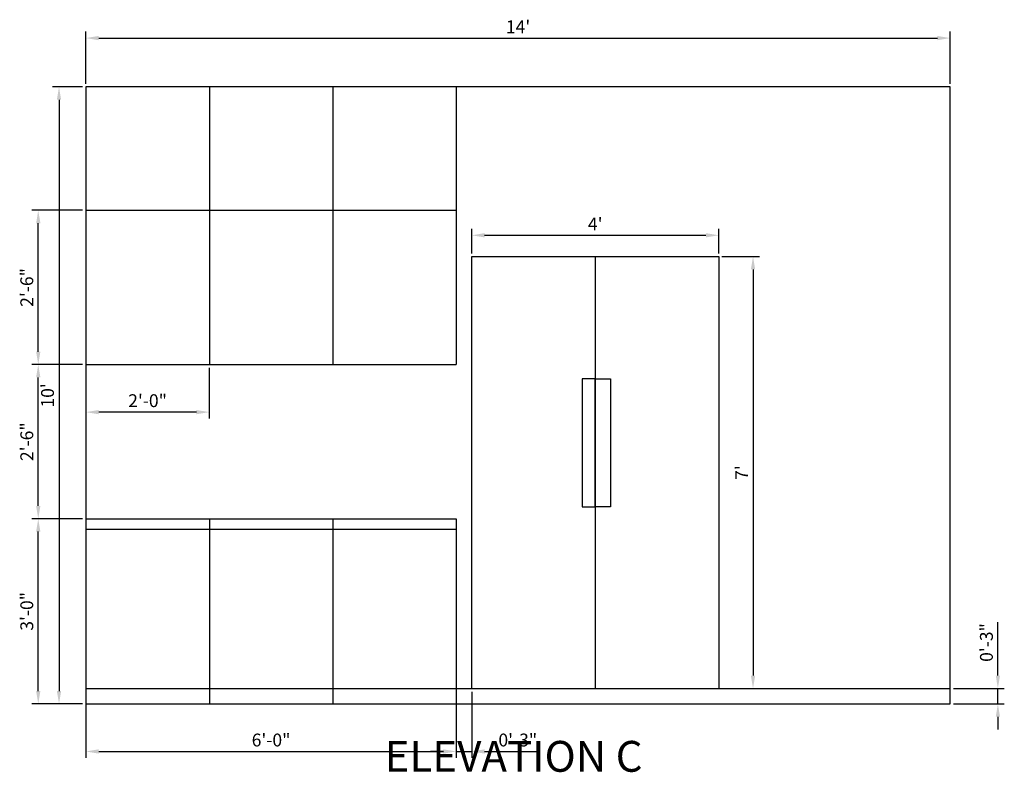
# Model space of a CAD drawing. Units: inches. Extents: x 125 to 951, y 142 to 358.
# Tile 4 of 4: x 759 to 951, y 210 to 356. Entities that reach past the tile are written whole.
import ezdxf

# ---------------------------------------------------------------- set-up
doc = ezdxf.new("R2010")
doc.units = ezdxf.units.IN
for name, color, linetype, lineweight in [('A-ANNO-DIMS', 2, 'Continuous', 18), ('A-ANNO-TEXT', 7, 'Continuous', 25), ('A-ELEV', 7, 'Continuous', 25), ('A-EQPM', 8, 'Continuous', 25), ('A-FLOR-CASE', 32, 'Continuous', 25), ('A-FLOR-CNTR', 30, 'Continuous', 25)]:
    doc.layers.add(name, color=color, linetype=linetype, lineweight=lineweight)
doc.styles.get("Standard").update_dxf_attribs({"font": 'arial.ttf'})
doc.dimstyles.new('ISO-25', dxfattribs={"dimtxt": 2.5, "dimasz": 2.5, "dimexe": 1.25, "dimexo": 0.625, "dimtad": 1, "dimlunit": 3, "dimtxsty": 'Standard', "dimcen": 2.5, "dimadec": 0, "dimazin": 0, "dimtfac": 1, "dimtmove": 0, "dimatfit": 3, "dimfxl": 1, "dimarcsym": 0})

# ---------------------------------------------------------------- blocks, each defined once
blk = doc.blocks.new('*D7')
at = {"layer": 'A-ANNO-DIMS', "color": 0, "lineweight": -2, "transparency": 16777216}
for p, q in [((771.42, 342.83), (765.58, 342.83)), ((766.83, 340.33), (766.83, 225.33)), ((771.42, 222.83), (765.58, 222.83))]:
    blk.add_line(p, q, dxfattribs=at)
at = {"layer": 'A-ANNO-DIMS', "color": 0, "transparency": 16777216}
for points in [[(766.41, 340.33), (767.24, 340.33), (766.83, 342.83)], [(766.41, 225.33), (767.24, 225.33), (766.83, 222.83)]]:
    blk.add_solid(points, dxfattribs=at)
at = {"layer": 'Defpoints', "color": 0, "transparency": 16777216}
for p in [(772.04, 342.83), (766.83, 222.83), (772.04, 222.83)]:
    blk.add_point(p, dxfattribs=at)
at = {"layer": 'A-ANNO-DIMS', "color": 0, "transparency": 16777216, "insert": (764.92, 282.83), "char_height": 2.5, "attachment_point": 5, "rotation": 90}
blk.add_mtext("10'", dxfattribs=at)
blk = doc.blocks.new('*D8')
at = {"layer": 'A-ANNO-DIMS', "color": 0, "lineweight": -2, "transparency": 16777216}
for p, q in [((772.04, 343.45), (772.04, 353.58)), ((774.54, 352.33), (937.54, 352.33)), ((940.04, 343.45), (940.04, 353.58))]:
    blk.add_line(p, q, dxfattribs=at)
at = {"layer": 'A-ANNO-DIMS', "color": 0, "transparency": 16777216}
for points in [[(774.54, 352.74), (774.54, 351.91), (772.04, 352.33)], [(937.54, 352.74), (937.54, 351.91), (940.04, 352.33)]]:
    blk.add_solid(points, dxfattribs=at)
at = {"layer": 'Defpoints', "color": 0, "transparency": 16777216}
for p in [(940.04, 352.33), (772.04, 342.83), (940.04, 342.83)]:
    blk.add_point(p, dxfattribs=at)
at = {"layer": 'A-ANNO-DIMS', "color": 0, "transparency": 16777216, "insert": (856.04, 354.21), "char_height": 2.5, "attachment_point": 5}
blk.add_mtext("14'", dxfattribs=at)
blk = doc.blocks.new('*D9')
at = {"layer": 'A-ANNO-DIMS', "color": 0, "lineweight": -2, "transparency": 16777216}
for p, q in [((895.67, 309.83), (902.96, 309.83)), ((901.71, 307.33), (901.71, 228.33)), ((895.67, 225.83), (902.96, 225.83))]:
    blk.add_line(p, q, dxfattribs=at)
at = {"layer": 'A-ANNO-DIMS', "color": 0, "transparency": 16777216}
for points in [[(901.29, 307.33), (902.12, 307.33), (901.71, 309.83)], [(901.29, 228.33), (902.12, 228.33), (901.71, 225.83)]]:
    blk.add_solid(points, dxfattribs=at)
at = {"layer": 'Defpoints', "color": 0, "transparency": 16777216}
for p in [(895.04, 309.83), (895.04, 225.83), (901.71, 225.83)]:
    blk.add_point(p, dxfattribs=at)
at = {"layer": 'A-ANNO-DIMS', "color": 0, "transparency": 16777216, "insert": (899.83, 267.83), "char_height": 2.5, "attachment_point": 5, "rotation": 90}
blk.add_mtext("7'", dxfattribs=at)
blk = doc.blocks.new('*D10')
at = {"layer": 'A-ANNO-DIMS', "color": 0, "lineweight": -2, "transparency": 16777216}
for p, q in [((847.04, 310.45), (847.04, 315.22)), ((849.54, 313.97), (892.54, 313.97)), ((895.04, 310.45), (895.04, 315.22))]:
    blk.add_line(p, q, dxfattribs=at)
at = {"layer": 'A-ANNO-DIMS', "color": 0, "transparency": 16777216}
for points in [[(849.54, 314.39), (849.54, 313.56), (847.04, 313.97)], [(892.54, 314.39), (892.54, 313.56), (895.04, 313.97)]]:
    blk.add_solid(points, dxfattribs=at)
at = {"layer": 'Defpoints', "color": 0, "transparency": 16777216}
for p in [(895.04, 313.97), (847.04, 309.83), (895.04, 309.83)]:
    blk.add_point(p, dxfattribs=at)
at = {"layer": 'A-ANNO-DIMS', "color": 0, "transparency": 16777216, "insert": (871.04, 315.85), "char_height": 2.5, "attachment_point": 5}
blk.add_mtext("4'", dxfattribs=at)
blk = doc.blocks.new('*D65')
at = {"layer": 'A-ANNO-DIMS', "color": 0, "lineweight": -2, "transparency": 16777216}
for p, q in [((772.04, 225.2), (772.04, 212.33)), ((844.04, 225.2), (844.04, 212.33)), ((774.54, 213.58), (841.54, 213.58))]:
    blk.add_line(p, q, dxfattribs=at)
at = {"layer": 'A-ANNO-DIMS', "color": 0, "transparency": 16777216}
for points in [[(774.54, 213.99), (774.54, 213.16), (772.04, 213.58)], [(841.54, 213.99), (841.54, 213.16), (844.04, 213.58)]]:
    blk.add_solid(points, dxfattribs=at)
at = {"layer": 'Defpoints', "color": 0, "transparency": 16777216}
for p in [(772.04, 225.83), (844.04, 225.83), (844.04, 213.58)]:
    blk.add_point(p, dxfattribs=at)
at = {"layer": 'A-ANNO-DIMS', "color": 0, "transparency": 16777216, "insert": (808.04, 215.48), "char_height": 2.5, "attachment_point": 5}
blk.add_mtext('6\'-0"', dxfattribs=at)
blk = doc.blocks.new('*D66')
at = {"layer": 'A-ANNO-DIMS', "color": 0, "lineweight": -2, "transparency": 16777216}
for p, q in [((844.04, 225.2), (844.04, 212.33)), ((847.04, 225.2), (847.04, 212.33)), ((841.54, 213.58), (839.04, 213.58)), ((844.04, 213.58), (847.04, 213.58)), ((849.54, 213.58), (859.94, 213.58))]:
    blk.add_line(p, q, dxfattribs=at)
at = {"layer": 'A-ANNO-DIMS', "color": 0, "transparency": 16777216}
for points in [[(841.54, 213.99), (841.54, 213.16), (844.04, 213.58)], [(849.54, 213.99), (849.54, 213.16), (847.04, 213.58)]]:
    blk.add_solid(points, dxfattribs=at)
at = {"layer": 'Defpoints', "color": 0, "transparency": 16777216}
for p in [(844.04, 225.83), (847.04, 225.83), (847.04, 213.58)]:
    blk.add_point(p, dxfattribs=at)
at = {"layer": 'A-ANNO-DIMS', "color": 0, "transparency": 16777216, "insert": (855.99, 215.48), "char_height": 2.5, "attachment_point": 5}
blk.add_mtext('0\'-3"', dxfattribs=at)
blk = doc.blocks.new('*D67')
at = {"layer": 'A-ANNO-DIMS', "color": 0, "lineweight": -2, "transparency": 16777216}
for p, q in [((771.42, 258.83), (761.54, 258.83)), ((762.79, 225.33), (762.79, 256.33)), ((771.42, 222.83), (761.54, 222.83))]:
    blk.add_line(p, q, dxfattribs=at)
at = {"layer": 'A-ANNO-DIMS', "color": 0, "transparency": 16777216}
for points in [[(762.38, 256.33), (763.21, 256.33), (762.79, 258.83)], [(762.38, 225.33), (763.21, 225.33), (762.79, 222.83)]]:
    blk.add_solid(points, dxfattribs=at)
at = {"layer": 'Defpoints', "color": 0, "transparency": 16777216}
for p in [(762.79, 258.83), (772.04, 258.83), (772.04, 222.83)]:
    blk.add_point(p, dxfattribs=at)
at = {"layer": 'A-ANNO-DIMS', "color": 0, "transparency": 16777216, "insert": (760.89, 240.83), "char_height": 2.5, "attachment_point": 5, "rotation": 90}
blk.add_mtext('3\'-0"', dxfattribs=at)
blk = doc.blocks.new('*D68')
at = {"layer": 'A-ANNO-DIMS', "color": 0, "lineweight": -2, "transparency": 16777216}
for p, q in [((771.42, 288.83), (761.54, 288.83)), ((762.79, 261.33), (762.79, 286.33)), ((771.42, 258.83), (761.54, 258.83))]:
    blk.add_line(p, q, dxfattribs=at)
at = {"layer": 'A-ANNO-DIMS', "color": 0, "transparency": 16777216}
for points in [[(762.38, 286.33), (763.21, 286.33), (762.79, 288.83)], [(762.38, 261.33), (763.21, 261.33), (762.79, 258.83)]]:
    blk.add_solid(points, dxfattribs=at)
at = {"layer": 'Defpoints', "color": 0, "transparency": 16777216}
for p in [(762.79, 288.83), (772.04, 288.83), (772.04, 258.83)]:
    blk.add_point(p, dxfattribs=at)
at = {"layer": 'A-ANNO-DIMS', "color": 0, "transparency": 16777216, "insert": (760.89, 273.83), "char_height": 2.5, "attachment_point": 5, "rotation": 90}
blk.add_mtext('2\'-6"', dxfattribs=at)
blk = doc.blocks.new('*D69')
at = {"layer": 'A-ANNO-DIMS', "color": 0, "lineweight": -2, "transparency": 16777216}
for p, q in [((771.42, 318.83), (761.54, 318.83)), ((762.79, 291.33), (762.79, 316.33)), ((771.42, 288.83), (761.54, 288.83))]:
    blk.add_line(p, q, dxfattribs=at)
at = {"layer": 'A-ANNO-DIMS', "color": 0, "transparency": 16777216}
for points in [[(762.38, 316.33), (763.21, 316.33), (762.79, 318.83)], [(762.38, 291.33), (763.21, 291.33), (762.79, 288.83)]]:
    blk.add_solid(points, dxfattribs=at)
at = {"layer": 'Defpoints', "color": 0, "transparency": 16777216}
for p in [(762.79, 318.83), (772.04, 318.83), (772.04, 288.83)]:
    blk.add_point(p, dxfattribs=at)
at = {"layer": 'A-ANNO-DIMS', "color": 0, "transparency": 16777216, "insert": (760.89, 303.83), "char_height": 2.5, "attachment_point": 5, "rotation": 90}
blk.add_mtext('2\'-6"', dxfattribs=at)
blk = doc.blocks.new('*D70')
at = {"layer": 'A-ANNO-DIMS', "color": 0, "lineweight": -2, "transparency": 16777216}
for p, q in [((772.04, 288.2), (772.04, 278.33)), ((796.04, 288.2), (796.04, 278.33)), ((793.54, 279.58), (774.54, 279.58))]:
    blk.add_line(p, q, dxfattribs=at)
at = {"layer": 'A-ANNO-DIMS', "color": 0, "transparency": 16777216}
for points in [[(774.54, 279.99), (774.54, 279.16), (772.04, 279.58)], [(793.54, 279.99), (793.54, 279.16), (796.04, 279.58)]]:
    blk.add_solid(points, dxfattribs=at)
at = {"layer": 'Defpoints', "color": 0, "transparency": 16777216}
for p in [(772.04, 288.83), (796.04, 288.83), (772.04, 279.58)]:
    blk.add_point(p, dxfattribs=at)
at = {"layer": 'A-ANNO-DIMS', "color": 0, "transparency": 16777216, "insert": (784.04, 281.48), "char_height": 2.5, "attachment_point": 5}
blk.add_mtext('2\'-0"', dxfattribs=at)
blk = doc.blocks.new('*D71')
at = {"layer": 'A-ANNO-DIMS', "color": 0, "lineweight": -2, "transparency": 16777216}
for p, q in [((949.29, 228.33), (949.29, 238.72)), ((940.67, 225.83), (950.54, 225.83)), ((949.29, 222.83), (949.29, 225.83)), ((940.67, 222.83), (950.54, 222.83)), ((949.29, 220.33), (949.29, 217.83))]:
    blk.add_line(p, q, dxfattribs=at)
at = {"layer": 'A-ANNO-DIMS', "color": 0, "transparency": 16777216}
for points in [[(948.88, 228.33), (949.71, 228.33), (949.29, 225.83)], [(948.88, 220.33), (949.71, 220.33), (949.29, 222.83)]]:
    blk.add_solid(points, dxfattribs=at)
at = {"layer": 'Defpoints', "color": 0, "transparency": 16777216}
for p in [(940.04, 225.83), (949.29, 225.83), (940.04, 222.83)]:
    blk.add_point(p, dxfattribs=at)
at = {"layer": 'A-ANNO-DIMS', "color": 0, "transparency": 16777216, "insert": (947.39, 234.77), "char_height": 2.5, "attachment_point": 5, "rotation": 90}
blk.add_mtext('0\'-3"', dxfattribs=at)

msp = doc.modelspace()

# ---------------------------------------------------------------- linework, layer by layer
at = {"layer": 'A-ELEV'}
for p, q in [((772.042, 342.827), (772.042, 222.827)), ((940.042, 342.827), (772.042, 342.827)), ((940.042, 222.827), (940.042, 342.827)), ((772.042, 222.827), (940.042, 222.827))]:
    msp.add_line(p, q, dxfattribs=at)
at = {"layer": 'A-EQPM'}
for p, q in [((847.042, 225.827), (847.042, 309.827)), ((847.042, 309.827), (895.042, 309.827)), ((871.042, 309.827), (871.042, 225.827)), ((895.042, 309.827), (895.042, 225.827))]:
    msp.add_line(p, q, dxfattribs=at)
for points in [[(871.042, 286.049), (868.497, 286.049), (868.497, 261.135), (871.042, 261.135)], [(871.042, 286.049), (874.017, 286.049), (874.017, 261.135), (871.042, 261.135)]]:
    msp.add_lwpolyline(points, close=True, dxfattribs=at)
at = {"layer": 'A-FLOR-CASE'}
for p, q in [((796.042, 342.827), (796.042, 288.827)), ((820.042, 342.827), (820.042, 288.827)), ((844.042, 342.827), (844.042, 288.827)), ((772.042, 318.827), (844.042, 318.827)), ((772.042, 288.827), (844.042, 288.827)), ((796.042, 258.827), (796.042, 222.827)), ((820.042, 258.827), (820.042, 222.827)), ((844.042, 258.827), (844.042, 222.827)), ((772.042, 225.827), (940.042, 225.827)), ((844.042, 225.827), (847.042, 225.827))]:
    msp.add_line(p, q, dxfattribs=at)
at = {"layer": 'A-FLOR-CNTR'}
for p, q in [((772.042, 258.827), (844.042, 258.827)), ((772.042, 256.827), (844.042, 256.827))]:
    msp.add_line(p, q, dxfattribs=at)

# ---------------------------------------------------------------- texts
at = {"layer": 'A-ANNO-TEXT', "insert": (830.116, 215.627), "char_height": 6, "attachment_point": 1}
msp.add_mtext_dynamic_manual_height_columns('ELEVATION C', width=61.9198, gutter_width=12.5, heights=[3.837], dxfattribs=at)

# ---------------------------------------------------------------- dimensions: what is measured, and where the dimension line sits
at = {"layer": 'A-ANNO-DIMS'}
for base, p1, p2, override, picture, middle in [((940.042, 352.325), (772.042, 342.827), (940.042, 342.827), {"dimclrd": 0, "dimclre": 0, "dimclrt": 0}, '*D8', (856.042, 354.205)), ((895.042, 313.973), (847.042, 309.827), (895.042, 309.827), {"dimclrd": 0, "dimclre": 0, "dimclrt": 0}, '*D10', (871.042, 315.848)), ((844.042, 213.577), (772.042, 225.827), (844.042, 225.827), {"dimdec": 1, "dimlfac": 1, "dimrnd": 0, "dimzin": 1, "dimdsep": 46, "dimlunit": 4, "dimfrac": 2}, '*D65', (808.042, 215.478)), ((847.042, 213.577), (844.042, 225.827), (847.042, 225.827), {"dimdec": 1, "dimlfac": 1, "dimrnd": 0, "dimzin": 1, "dimdsep": 46, "dimlunit": 4, "dimfrac": 2}, '*D66', (855.99, 215.479))]:
    dim = msp.add_linear_dim(base=base, p1=p1, p2=p2, dimstyle='ISO-25', override=override, dxfattribs=at)
    dim.commit()
    dim.dimension.update_dxf_attribs({"geometry": picture, "text_midpoint": middle})
for base, p1, p2, angle, override, picture, middle in [((766.825, 222.827), (772.042, 342.827), (772.042, 222.827), 90, {"dimclrd": 0, "dimclre": 0, "dimclrt": 0}, '*D7', (764.924, 282.827)), ((762.792, 318.827), (772.042, 288.827), (772.042, 318.827), 90, {"dimdec": 1, "dimlfac": 1, "dimrnd": 0, "dimzin": 1, "dimdsep": 46, "dimlunit": 4, "dimfrac": 2}, '*D69', (760.89, 303.827)), ((901.707, 225.827), (895.042, 309.827), (895.042, 225.827), 90, {"dimclrd": 0, "dimclre": 0, "dimclrt": 0}, '*D9', (899.832, 267.827)), ((762.792, 288.827), (772.042, 258.827), (772.042, 288.827), 90, {"dimdec": 1, "dimlfac": 1, "dimrnd": 0, "dimzin": 1, "dimdsep": 46, "dimlunit": 4, "dimfrac": 2}, '*D68', (760.89, 273.827)), ((772.042, 279.577), (796.042, 288.827), (772.042, 288.827), 180, {"dimdec": 1, "dimlfac": 1, "dimrnd": 0, "dimzin": 1, "dimdsep": 46, "dimlunit": 4, "dimfrac": 2}, '*D70', (784.042, 281.478)), ((762.792, 258.827), (772.042, 222.827), (772.042, 258.827), 90, {"dimdec": 1, "dimlfac": 1, "dimrnd": 0, "dimzin": 1, "dimdsep": 46, "dimlunit": 4, "dimfrac": 2}, '*D67', (760.89, 240.827)), ((949.292, 225.827), (940.042, 222.827), (940.042, 225.827), 90, {"dimdec": 1, "dimlfac": 1, "dimrnd": 0, "dimzin": 1, "dimdsep": 46, "dimlunit": 4, "dimfrac": 2}, '*D71', (947.39, 234.775))]:
    dim = msp.add_linear_dim(base=base, p1=p1, p2=p2, angle=angle, dimstyle='ISO-25', override=override, dxfattribs=at)
    dim.commit()
    dim.dimension.update_dxf_attribs({"geometry": picture, "text_midpoint": middle})

doc.saveas('drawing.dxf')
